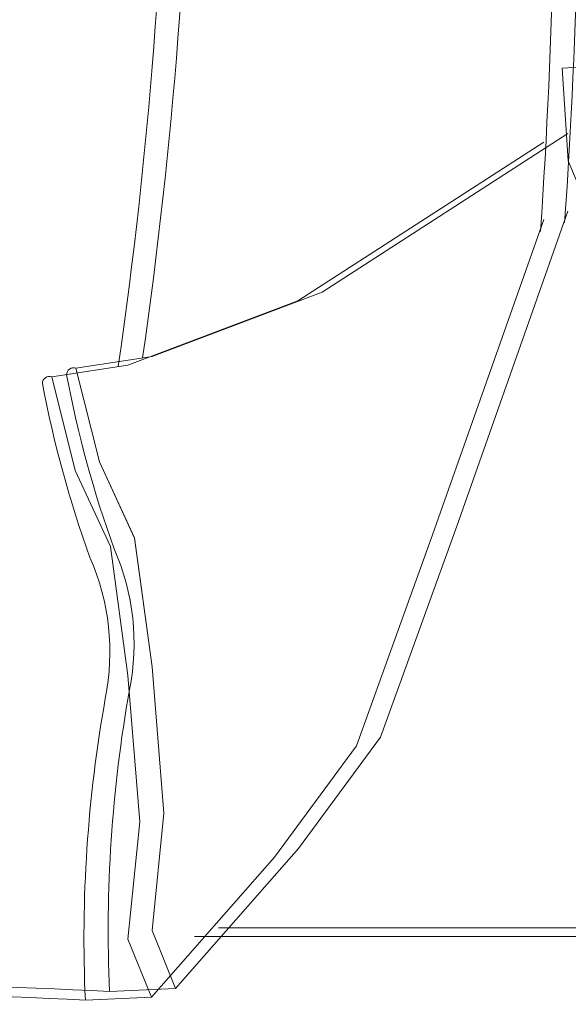
# Model space of a CAD drawing. Units: inches. Extents: x 1901 to 2863, y 888 to 2433.
# Tile 43 of 91: x 2710 to 2726, y 1566 to 1595. Entities that reach past the tile are written whole.
import ezdxf

# ---------------------------------------------------------------- set-up
doc = ezdxf.new("R2010")
doc.units = ezdxf.units.IN
doc.layers.add('A-FURN', color=8, linetype='Continuous', lineweight=18)

# ---------------------------------------------------------------- blocks, each defined once
blk = doc.blocks.new('BED-DOUBLE')
for p, q in [((33.854, 59.666), (31.896, 59.577, 4.346)), ((33.854, 59.666), (31.896, 59.577, 4.346)), ((31.896, 59.577), (28.246, 55.417)), ((31.896, 59.577), (28.246, 55.417)), ((33.137, 59.41), (31.178, 59.321, 4.346)), ((33.137, 59.41), (31.178, 59.32, 4.346)), ((32.591, 57.851), (31.896, 59.577)), ((32.591, 57.851), (31.896, 59.577)), ((31.178, 59.321), (27.529, 55.161)), ((31.178, 59.32), (27.529, 55.16)), ((31.873, 57.595), (31.178, 59.321)), ((31.873, 57.595), (31.178, 59.32)), ((0.744, 57.778), (30.62, 57.778)), ((0.744, 57.778), (30.62, 57.778)), ((31.525, 54.117), (31.873, 57.595)), ((31.525, 54.117), (31.873, 57.595)), ((32.243, 54.374), (32.591, 57.851)), ((32.243, 54.373), (32.591, 57.851)), ((28.246, 55.417), (25.814, 52.113)), ((28.246, 55.417), (25.814, 52.113)), ((27.529, 55.161), (25.096, 51.857)), ((27.529, 55.16), (25.096, 51.856)), ((31.873, 49.77), (31.525, 54.117)), ((31.873, 49.77), (31.525, 54.117)), ((32.591, 50.027), (32.243, 54.374)), ((32.591, 50.026), (32.243, 54.373)), ((25.814, 52.113), (23.554, 45.853)), ((25.814, 52.113), (23.554, 45.853)), ((25.096, 51.857), (22.837, 45.597)), ((25.096, 51.856), (22.837, 45.597)), ((33.112, 46.201), (32.591, 50.027)), ((33.112, 46.201), (32.591, 50.026)), ((32.394, 45.945), (31.873, 49.77)), ((32.394, 45.944), (31.873, 49.77)), ((34.155, 43.941), (33.112, 46.201)), ((34.155, 43.94), (33.112, 46.201)), ((33.437, 43.684), (32.394, 45.945)), ((33.437, 43.684), (32.394, 45.944)), ((23.554, 45.853), (20.261, 36.492)), ((23.554, 45.853), (20.261, 36.491)), ((22.837, 45.597), (19.543, 36.235)), ((22.837, 45.597), (19.543, 36.235)), ((34.85, 41.158), (34.155, 43.941)), ((34.85, 41.158), (34.155, 43.94)), ((34.132, 40.902), (33.437, 43.684)), ((34.132, 40.902), (33.437, 43.684)), ((32.591, 40.811), (34.85, 41.158)), ((32.591, 40.81), (34.85, 41.158)), ((27.551, 38.898), (32.591, 40.811)), ((27.551, 38.898), (32.591, 40.81)), ((31.873, 40.554), (34.132, 40.902)), ((31.873, 40.554), (34.132, 40.902)), ((26.834, 38.642), (31.873, 40.554)), ((26.834, 38.641), (31.873, 40.554)), ((20.261, 34.194), (27.551, 38.898)), ((20.261, 34.193), (27.551, 38.898)), ((19.543, 33.937), (26.834, 38.642)), ((19.543, 33.937), (26.834, 38.641)), ((19.538, 34.745), (18.096, 38.192)), ((19.538, 34.745), (18.096, 38.192)), ((19.71, 31.991), (19.538, 34.745)), ((19.71, 31.991), (19.538, 34.745)), ((16.706, 31.803), (19.71, 31.991)), ((16.706, 31.803), (19.71, 31.991))]:
    blk.add_line(p, q)
for centre, radius, start, end in [((-6.729, 57.848), 40.624, 349.8763, 2.5657), ((-6.729, 57.847), 40.624, 349.8763, 2.5657), ((41.517, 204.859), 145.395, 266.97912, 273.83645), ((41.517, 204.859), 145.395, 266.97912, 273.83645), ((-7.447, 57.591), 40.624, 349.8763, 2.5657), ((-7.447, 57.591), 40.624, 349.8763, 2.5657), ((40.799, 204.603), 145.395, 266.97912, 273.83645), ((40.799, 204.602), 145.395, 266.97912, 273.83645), ((40.115, 49.333), 6.988, 168.6608, 203.7384), ((40.115, 49.333), 6.988, 168.6608, 203.7384), ((39.397, 49.077), 6.988, 168.6608, 203.7384), ((39.397, 49.076), 6.988, 168.6608, 203.7384), ((2.408, 35.198), 33.294, 10.6617, 19.8806), ((2.408, 35.198), 33.294, 10.6617, 19.8806), ((1.69, 34.942), 33.294, 10.6617, 19.8806), ((1.69, 34.941), 33.294, 10.6617, 19.8806), ((34.92, 41.353), 0.207, 250.2464, 1.1377), ((34.92, 41.353), 0.207, 250.2464, 1.1377), ((34.202, 41.097), 0.207, 250.2464, 1.1377), ((34.202, 41.097), 0.207, 250.2464, 1.1377), ((176.248, 20.155), 144.857, 171.78449, 186.90062), ((176.248, 20.155), 144.857, 171.78449, 186.90062), ((175.53, 19.899), 144.857, 171.78449, 186.90062), ((175.53, 19.899), 144.857, 171.78449, 186.90062), ((205.143, 24.201), 185.219, 176.08655, 186.78213), ((205.143, 24.2), 185.219, 176.08655, 186.78213), ((204.426, 23.944), 185.219, 176.08655, 186.78213), ((204.426, 23.944), 185.219, 176.08655, 186.78213)]:
    blk.add_arc(centre, radius, start, end)

msp = doc.modelspace()

# ---------------------------------------------------------------- linework, layer by layer
at = {"layer": 'A-FURN'}
msp.add_line((2745.864, 1568.498), (2715.987, 1568.498), dxfattribs=at)
msp.add_line((2745.864, 1568.498), (2715.987, 1568.498), dxfattribs=at)

# ---------------------------------------------------------------- block references
at = {"layer": 'A-FURN', "rotation": 180}
msp.add_blockref('BED-DOUBLE', (2745.89, 1626.019), dxfattribs=at)

doc.saveas('drawing.dxf')
